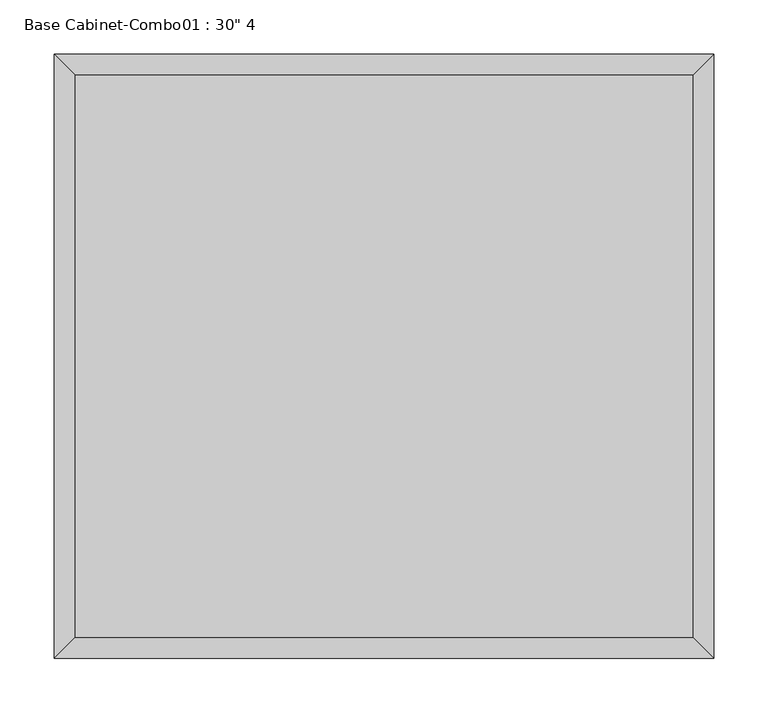
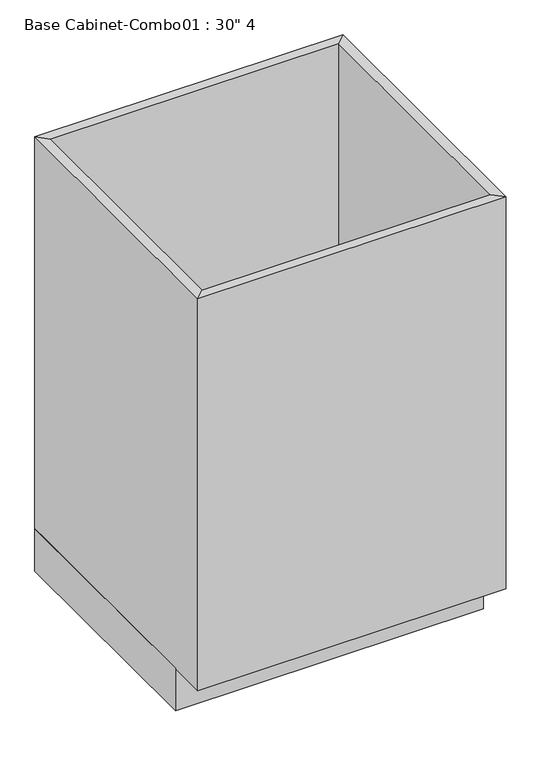
"""IFC4 building model written with IfcOpenShell, lengths in millimetres: furniture geometry."""

from ifc_helpers import new_model, si_unit, frame, origin, origin_with_axes, place, context, project, spatial, polyline, outline, extrude, faceted_brep, source, transform, mapped, element, save


def furniture_6369f5ad(model_context):
    return source(origin(), model_context, "Body", "SolidModel", [
        extrude(outline(polyline([(323.5377049, 0.0), (323.5377049, -482.6), (-286.0622951, -482.6), (-286.0622951, 0.0), (323.5377049, 0.0)])), origin_with_axes(), (0.0, 0.0, 1.0), 88.9),
        faceted_brep([(304.4877049, -539.75, 908.05), (304.4877049, -539.75, 88.9), (-267.0122951, -539.75, 88.9), (-267.0122951, -539.75, 908.05), (323.5377049, -558.8, 908.05), (-286.0622951, -558.8, 908.05), (323.5377049, -558.8, 88.9), (-286.0622951, -558.8, 88.9), (-267.0122951, -19.05, 88.9), (-267.0122951, -19.05, 908.05), (-286.0622951, 0.0, 908.05), (-286.0622951, 0.0, 88.9), (304.4877049, -19.05, 88.9), (304.4877049, -19.05, 908.05), (323.5377049, 0.0, 908.05), (323.5377049, 0.0, 88.9)], [[[0, 1, 2, 3]], [[4, 0, 3, 5]], [[6, 4, 5, 7]], [[1, 6, 7, 2]], [[3, 2, 8, 9]], [[5, 3, 9, 10]], [[7, 5, 10, 11]], [[2, 7, 11, 8]], [[9, 8, 12, 13]], [[10, 9, 13, 14]], [[11, 10, 14, 15]], [[8, 11, 15, 12]], [[13, 12, 1, 0]], [[14, 13, 0, 4]], [[15, 14, 4, 6]], [[12, 15, 6, 1]]]),
        extrude(outline(polyline([(304.4877049, -19.05), (304.4877049, -539.75), (-267.0122951, -539.75), (-267.0122951, -19.05), (304.4877049, -19.05)])), frame((0.0, 0.0, 88.9), z_axis=(0.0, 0.0, 1.0), x_axis=(1.0, 0.0, 0.0)), (0.0, 0.0, 1.0), 19.05),
    ])


if __name__ == "__main__":
    model = new_model("IFC4")
    model_context = context("Model", 3, world=origin())
    ifc_project = project(units=[si_unit("LENGTHUNIT", "METRE", prefix="MILLI")], contexts=[model_context])
    site = spatial("IfcSite", under=ifc_project)
    building = spatial("IfcBuilding", under=site)
    placement = place(None, origin())
    furniture_shape = furniture_6369f5ad(model_context)
    element("IfcFurniture", 1, ObjectType="Base Cabinet-Combo01 : 30\" 4", at=placement, inside=building, context=model_context, shape_type="MappedRepresentation", body=[
        mapped(furniture_shape, transform((0.0, 0.0, 0.0), x_axis=(1.0, 0.0, 0.0), y_axis=(0.0, 1.0, 0.0), z_axis=(0.0, 0.0, 1.0))),
    ])
    save(model, "model.ifc")

# Revit data of these elements
# Type "Base Cabinet-Combo01 : 30\" 4"
#   Depth = 1' - 10"
#   Height = 2' - 11 3/4"
#   Toe Depth = 0' - 3"
#   Toe Height = 0' - 3 1/2"
#   Width = 2' - 0"
#   Default Elevation = 0
# Element 1 (IfcFurniture, "Base Cabinet-Combo01 : 30\" 4")
#   Materials on its faces: "Cabinet"
# Materials
#   "Cabinet": colour RGB 204 122 2, transparency 0
